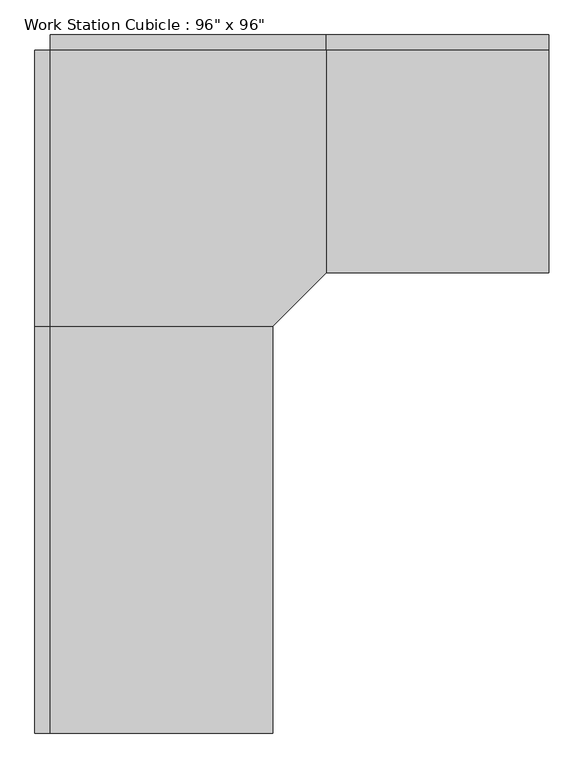
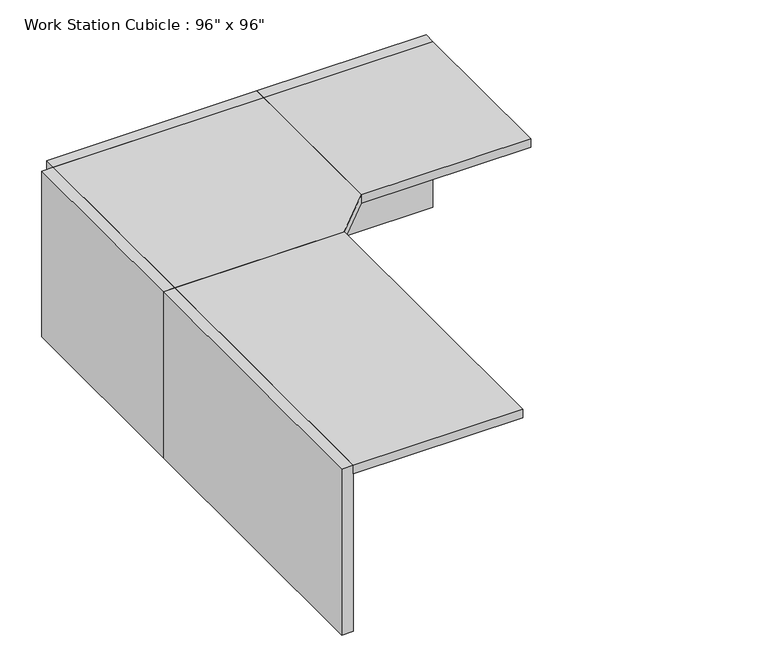
"""IFC4 building model written with IfcOpenShell, lengths in millimetres: furniture geometry."""

from ifc_helpers import new_model, si_unit, frame, origin, origin_with_axes, place, context, project, spatial, polyline, outline, extrude, source, transform, mapped, element, save


def furniture_cb58875c(model_context):
    return source(origin(), model_context, "Body", "SweptSolid", [
        extrude(outline(polyline([(-80.9317522, -545.8230076), (833.4682478, -545.8230076), (833.4682478, -1282.4230076), (655.6682478, -1460.2230076), (-80.9317522, -1460.2230076), (-80.9317522, -545.8230076)])), frame((0.0, 0.0, 723.9), z_axis=(0.0, 0.0, 1.0), x_axis=(1.0, 0.0, 0.0)), (0.0, 0.0, 1.0), 38.1),
        extrude(outline(polyline([(655.6682478, -2806.4230076), (-80.9317522, -2806.4230076), (-80.9317522, -1460.2230076), (655.6682478, -1460.2230076), (655.6682478, -2806.4230076)])), frame((0.0, 0.0, 723.9), z_axis=(0.0, 0.0, 1.0), x_axis=(1.0, 0.0, 0.0)), (0.0, 0.0, 1.0), 38.1),
        extrude(outline(polyline([(1570.0682478, -1282.4230076), (833.4682478, -1282.4230076), (833.4682478, -545.8230076), (1570.0682478, -545.8230076), (1570.0682478, -1282.4230076)])), frame((0.0, 0.0, 723.9), z_axis=(0.0, 0.0, 1.0), x_axis=(1.0, 0.0, 0.0)), (0.0, 0.0, 1.0), 38.1),
        extrude(outline(polyline([(1570.0682478, -545.8230076), (833.4682478, -545.8230076), (833.4682478, -495.0230076), (1570.0682478, -495.0230076), (1570.0682478, -545.8230076)])), origin_with_axes(), (0.0, 0.0, 1.0), 762.0),
        extrude(outline(polyline([(833.4682478, -545.8230076), (-80.9317522, -545.8230076), (-80.9317522, -495.0230076), (833.4682478, -495.0230076), (833.4682478, -545.8230076)])), origin_with_axes(), (0.0, 0.0, 1.0), 762.0),
        extrude(outline(polyline([(-80.9317522, -1460.2230076), (-131.7317522, -1460.2230076), (-131.7317522, -545.8230076), (-80.9317522, -545.8230076), (-80.9317522, -1460.2230076)])), origin_with_axes(), (0.0, 0.0, 1.0), 762.0),
        extrude(outline(polyline([(-80.9317522, -2806.4230076), (-131.7317522, -2806.4230076), (-131.7317522, -1460.2230076), (-80.9317522, -1460.2230076), (-80.9317522, -2806.4230076)])), origin_with_axes(), (0.0, 0.0, 1.0), 762.0),
    ])


if __name__ == "__main__":
    model = new_model("IFC4")
    model_context = context("Model", 3, world=origin())
    ifc_project = project(units=[si_unit("LENGTHUNIT", "METRE", prefix="MILLI")], contexts=[model_context])
    site = spatial("IfcSite", under=ifc_project)
    building = spatial("IfcBuilding", under=site)
    placement = place(None, origin())
    furniture_shape = furniture_cb58875c(model_context)
    element("IfcFurniture", 1, ObjectType="Work Station Cubicle : 96\" x 96\"", at=placement, inside=building, context=model_context, shape_type="MappedRepresentation", body=[
        mapped(furniture_shape, transform((0.0, 0.0, 0.0), x_axis=(1.0, 0.0, 0.0), y_axis=(0.0, 1.0, 0.0), z_axis=(0.0, 0.0, 1.0))),
    ])
    save(model, "model.ifc")

# Revit data of these elements
# Type "Work Station Cubicle : 96\" x 96\""
#   Assembly Code = "E2020"
#   Desktop Height = 2' - 6"
#   Desktop1 Width = 2' - 5"
#   Desktop2 Width = 2' - 5"
#   Panel Height = 2' - 6"
#   Panel1 Length = 4' - 5"
#   Panel2 Length = 2' - 5"
#   Cube Panel Material = Textile - Light Gray
#   Work Top Material = Laminate, Ivory, Matte
#   Default Elevation = 0
# Element 1 (IfcFurniture, "Work Station Cubicle : 96\" x 96\"")
#   Materials on its faces: "Textile - Light Gray", "Laminate, Ivory, Matte"
# Materials
#   "Textile - Light Gray": class "Fabric", colour RGB 204 204 204, transparency 0
#   "Laminate, Ivory, Matte": class "Plastic", colour RGB 247 247 239, transparency 0, Description = "Plastic Laminate - Ivory, Matte", Cost = 0
